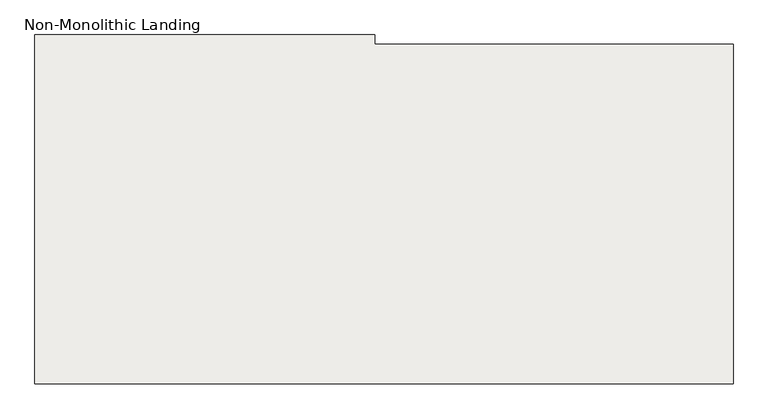
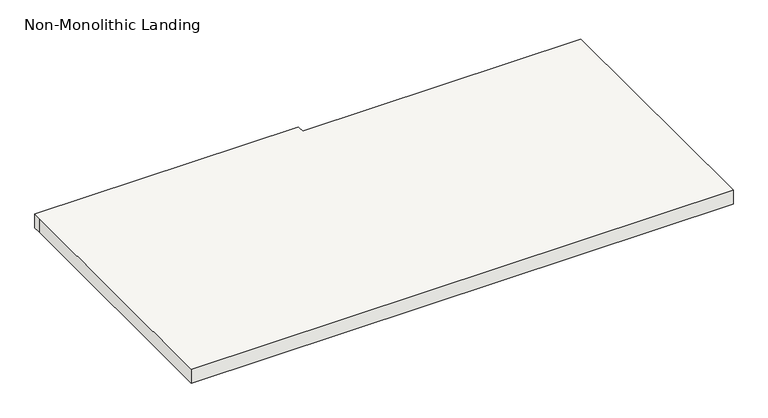
"""IFC4 building model written with IfcOpenShell, lengths in millimetres: slab geometry, Non-Monolithic Landing."""

from ifc_helpers import new_model, si_unit, origin, place, context, project, spatial, faceted_brep, source, transform, mapped, element, save


def non_monolithic_landing_a6268fe4(model_context):
    return source(origin(), model_context, "Body", "Brep", [
        faceted_brep([(-3400.7137331, -6527.0593836, 14204.2118174), (-3400.7137331, -6552.4593836, 14178.8118174), (-4315.1137331, -6552.4593836, 14178.8118174), (-4315.1137331, -6527.0593836, 14204.2118174), (-4365.9137331, -6527.0593836, 14223.2618174), (-4365.9137331, -6501.6593836, 14223.2618174), (-5280.3137331, -6501.6593836, 14223.2618174), (-5280.3137331, -6527.0593836, 14223.2618174), (-5280.3137331, -7441.4593836, 14223.2618174), (-3400.7137331, -7441.4593836, 14223.2618174), (-3400.7137331, -6527.0593836, 14223.2618174), (-4315.1137331, -6552.4593836, 14172.4618174), (-3400.7137331, -6552.4593836, 14172.4618174), (-3400.7137331, -7441.4593836, 14172.4618174), (-5280.3137331, -7441.4593836, 14172.4618174), (-5280.3137331, -6527.0593836, 14172.4618174), (-5280.3137331, -6501.6593836, 14172.4618174), (-4365.9137331, -6501.6593836, 14172.4618174), (-4365.9137331, -6527.0593836, 14172.4618174), (-4315.1137331, -6527.0593836, 14172.4618174)], [[[0, 1, 2, 3]], [[4, 5, 6, 7, 8, 9, 10]], [[11, 12, 13, 14, 15, 16, 17, 18, 19]], [[12, 11, 2, 1]], [[11, 19, 3, 2]], [[4, 10, 0, 3, 19, 18]], [[5, 4, 18, 17]], [[6, 5, 17, 16]], [[7, 6, 16, 15]], [[8, 7, 15, 14]], [[9, 8, 14, 13]], [[10, 9, 13, 12, 1, 0]]]),
    ])


if __name__ == "__main__":
    model = new_model("IFC4")
    model_context = context("Model", 3, world=origin())
    ifc_project = project(units=[si_unit("LENGTHUNIT", "METRE", prefix="MILLI")], contexts=[model_context])
    site = spatial("IfcSite", under=ifc_project)
    building = spatial("IfcBuilding", under=site)
    placement = place(None, origin())
    non_monolithic_landing_shape = non_monolithic_landing_a6268fe4(model_context)
    element("IfcSlab", 1, ObjectType="Non-Monolithic Landing", at=placement, inside=building, context=model_context, shape_type="MappedRepresentation", body=[
        mapped(non_monolithic_landing_shape, transform((0.0, 0.0, 0.0), x_axis=(1.0, 0.0, 0.0), y_axis=(0.0, 1.0, 0.0), z_axis=(0.0, 0.0, 1.0))),
    ])
    save(model, "model.ifc")
